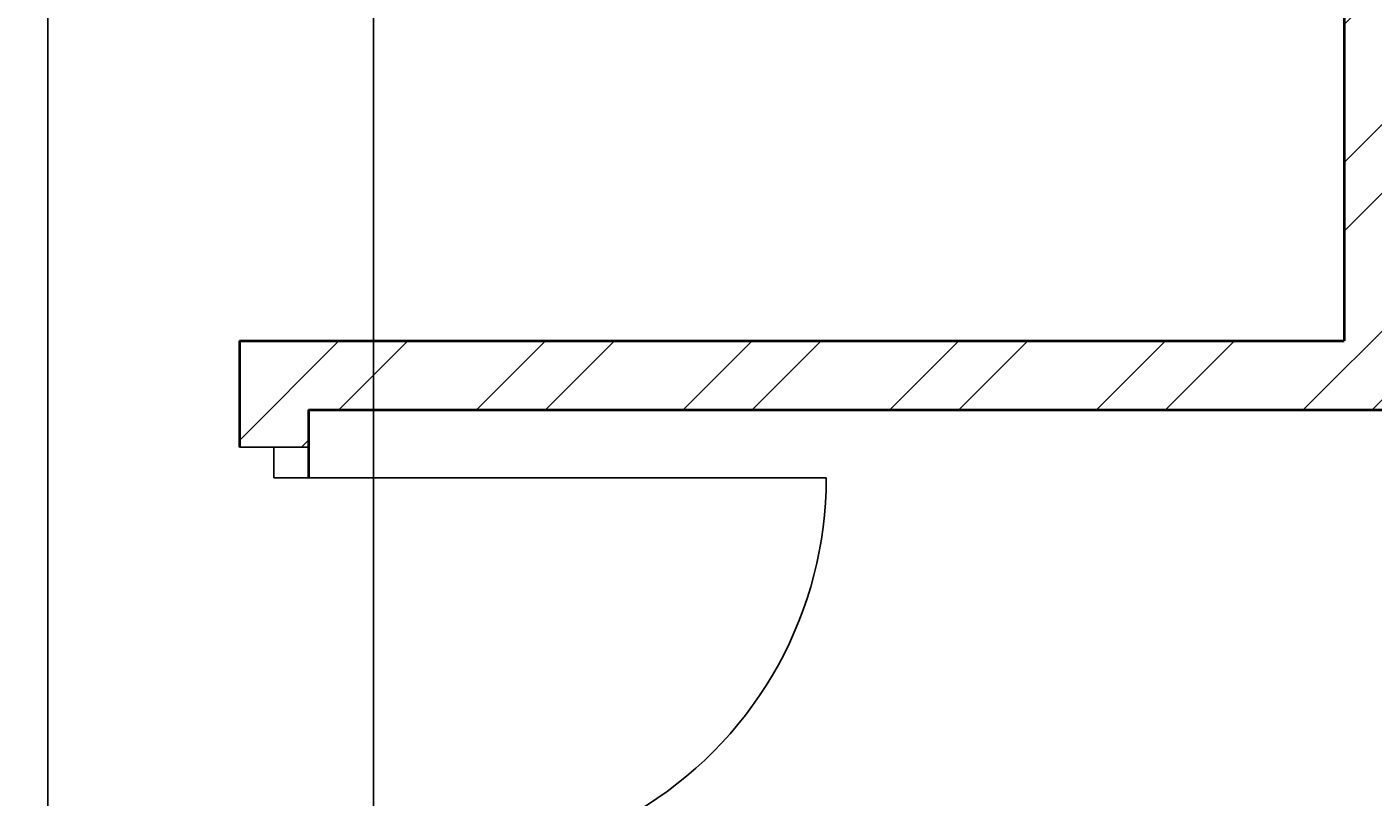
# Model space of a CAD drawing. Units: inches. Extents: x 2063 to 2617, y 1299 to 2210.
# Tile 17 of 22: x 2387 to 2475, y 1839 to 1889. Entities that reach past the tile are written whole.
import ezdxf

# ---------------------------------------------------------------- set-up
doc = ezdxf.new("R2010")
doc.units = ezdxf.units.IN
for name, color, linetype, lineweight in [('A-ANNO-DIMS', 2, 'Continuous', 18), ('A-DOOR', 11, 'Continuous', 25), ('A-WALL', 7, 'Continuous', 40)]:
    doc.layers.add(name, color=color, linetype=linetype, lineweight=lineweight)
doc.layers.add('A-WALL-PATT', color=215, linetype='Continuous', lineweight=13, true_color=0xa953a0)
doc.styles.get("Standard").update_dxf_attribs({"font": 'arial.ttf'})
doc.dimstyles.get("Standard").update_dxf_attribs({"dimtxt": 0.18, "dimasz": 0.18, "dimexe": 0.18, "dimexo": 0.0625, "dimgap": 0.09, "dimtad": 0, "dimtih": 1, "dimtoh": 1, "dimdec": 4, "dimzin": 0, "dimdsep": 46, "dimtxsty": 'Standard', "dimcen": 0.09, "dimadec": 0, "dimazin": 0, "dimtfac": 1, "dimtdec": 4, "dimtofl": 0, "dimtmove": 0, "dimatfit": 3, "dimfxl": 1, "dimtolj": 1, "dimtzin": 0, "dimarcsym": 0})

# ---------------------------------------------------------------- blocks, each defined once
blk = doc.blocks.new('*D55')
at = {"layer": 'A-ANNO-DIMS', "color": 0, "lineweight": -2, "transparency": 16777216}
for p, q in [((2388.15, 1975.75), (2388.15, 1317.702)), ((2409.375, 1975.75), (2409.375, 1317.702)), ((2388.33, 1317.882), (2398.297, 1317.882)), ((2409.195, 1317.882), (2399.229, 1317.882))]:
    blk.add_line(p, q, dxfattribs=at)
at = {"layer": 'A-ANNO-DIMS', "color": 0, "transparency": 16777216}
for points in [[(2388.33, 1317.912), (2388.33, 1317.852), (2388.15, 1317.882)], [(2409.195, 1317.912), (2409.195, 1317.852), (2409.375, 1317.882)]]:
    blk.add_solid(points, dxfattribs=at)
at = {"layer": 'Defpoints', "color": 0, "transparency": 16777216}
for p in [(2388.15, 1975.812), (2409.375, 1975.812), (2409.375, 1317.882)]:
    blk.add_point(p, dxfattribs=at)
at = {"layer": 'A-ANNO-DIMS', "color": 0, "transparency": 16777216, "insert": (2398.763, 1317.882), "char_height": 0.18, "attachment_point": 5}
blk.add_mtext('\\A1;21.225', dxfattribs=at)

msp = doc.modelspace()

# ---------------------------------------------------------------- hatches: boundary and pattern name
at = {"layer": 'A-WALL-PATT'}
h = msp.add_hatch(dxfattribs=at)
h.set_pattern_fill('ANSI32', color=256)
h.paths.add_polyline_path([(2553.6442, 2128.8122), (2511.1703, 2128.8122), (2511.1703, 2124.3122), (2549.1442, 2124.3122), (2549.1442, 2095.662), (2553.6442, 2095.662)])
h.paths.add_polyline_path([(2553.6442, 2035.662), (2549.1442, 2035.662), (2549.1442, 1980.3122), (2503.7214, 1980.3122), (2503.7214, 1975.8122), (2549.1442, 1975.8122), (2549.1442, 1962.9693), (2553.6442, 1962.9693)])
h.paths.add_polyline_path([(2553.6442, 1938.9693), (2549.1442, 1938.9693), (2549.1442, 1927.8122), (2477.1442, 1927.8122), (2477.1442, 1975.8122), (2481.2918, 1975.8122), (2481.2918, 1980.3122), (2453.2648, 1980.3122), (2453.2648, 1975.8122), (2472.6442, 1975.8122), (2472.6442, 1868.3122), (2400.6442, 1868.3122), (2400.6442, 1861.3782), (2405.1442, 1861.3782), (2405.1442, 1863.8122), (2480.9699, 1863.8122), (2480.9699, 1866.0622), (2480.9699, 1868.3122), (2477.1442, 1868.3122), (2477.1442, 1923.3122), (2549.1442, 1923.3122), (2549.1442, 1908.8504), (2553.6442, 1908.8504)])
h.paths.add_polyline_path([(2553.6442, 1884.8504), (2549.1442, 1884.8504), (2549.1442, 1868.3122), (2501.0636, 1868.3122), (2501.0636, 1863.8122), (2549.1442, 1863.8122), (2549.1442, 1826.0298), (2553.6442, 1826.0298)])
h.paths.add_polyline_path([(2388.1504, 1980.3122), (2340.6442, 1980.3122), (2340.6442, 2124.3122), (2358.7501, 2124.3122), (2358.7501, 2128.8122), (2316.3482, 2128.8122), (2316.3482, 2124.3122), (2336.1442, 2124.3122), (2336.1442, 1980.3122), (2289.1737, 1980.3122), (2289.1737, 1975.8122), (2336.1442, 1975.8122), (2336.1442, 1619.3122), (2333.1433, 1619.3122), (2333.1433, 1614.8122), (2344.1671, 1614.8122), (2344.1671, 1617.0622), (2344.1671, 1619.3122), (2340.6442, 1619.3122), (2340.6442, 1975.8122), (2388.1504, 1975.8122), (2388.1504, 1978.0622)])
h.paths.add_polyline_path([(2290.1442, 1614.8122), (2301.4594, 1614.8122), (2301.4594, 1617.0622), (2301.4594, 1619.3122), (2285.6442, 1619.3122), (2285.6442, 1566.8122), (2280.8619, 1566.8122), (2280.8619, 1564.5622), (2280.8619, 1562.3122), (2285.6442, 1562.3122), (2285.6442, 1442.3122), (2281.7879, 1442.3122), (2281.7879, 1437.8122), (2285.6442, 1437.8122), (2285.6442, 1401.8122), (2290.1442, 1401.8122)])
h.paths.add_polyline_path([(2549.1442, 1731.8122), (2405.1442, 1731.8122), (2405.1442, 1834.4638), (2402.8942, 1834.4638), (2400.6442, 1834.4638), (2400.6442, 1727.3122), (2549.1442, 1727.3122)])
h.paths.add_polyline_path([(2553.6442, 1766.0298), (2551.3942, 1766.0298), (2549.1442, 1766.0298), (2549.1442, 1686.7767), (2553.6442, 1686.7767)])
h.paths.add_polyline_path([(2553.6442, 1638.7767), (2551.3942, 1638.7767), (2549.1442, 1638.7767), (2549.1442, 1619.3122), (2448.6442, 1619.3122), (2448.6442, 1610.5671), (2450.8942, 1610.5671), (2453.1442, 1610.5671), (2453.1442, 1614.8122), (2549.1442, 1614.8122), (2549.1442, 1601.6421), (2553.6442, 1601.6421)])
h.paths.add_polyline_path([(2553.6442, 1577.6421), (2551.3942, 1577.6421), (2549.1442, 1577.6421), (2549.1442, 1566.8122), (2453.1442, 1566.8122), (2453.1442, 1591.5045), (2451.0335, 1591.5045), (2448.6442, 1591.5045), (2448.6442, 1566.8122), (2434.0475, 1566.8122), (2434.0475, 1562.3122), (2549.1442, 1562.3122), (2549.1442, 1533.48), (2553.6442, 1533.48)])
h.paths.add_polyline_path([(2553.6442, 1473.48), (2549.1442, 1473.48), (2549.1442, 1442.3122), (2502.6258, 1442.3122), (2502.6258, 1437.8122), (2549.1442, 1437.8122), (2549.1442, 1401.8122), (2553.6442, 1401.8122)])
h.paths.add_polyline_path([(2395.6442, 1562.3122), (2400.0901, 1562.3122), (2400.0901, 1564.5622), (2400.0901, 1566.8122), (2395.6442, 1566.8122), (2395.6442, 1619.3122), (2379.1127, 1619.3122), (2379.1127, 1614.8122), (2391.1442, 1614.8122), (2391.1442, 1401.8122), (2395.6442, 1401.8122), (2395.6442, 1437.8122), (2399.2425, 1437.8122), (2399.2425, 1440.0622), (2399.2425, 1442.3122), (2395.6442, 1442.3122)])
h.paths.add_polyline_path([(2442.6258, 1442.3122), (2419.6262, 1442.3122), (2419.6262, 1437.8122), (2442.6258, 1437.8122), (2442.6258, 1440.0622)])
h.paths.add_polyline_path([(2127.6442, 1480.2532), (2125.3942, 1480.2532), (2123.1442, 1480.2532), (2123.1442, 1401.8122), (2127.6442, 1401.8122), (2127.6442, 1437.8122), (2145.1538, 1437.8122), (2145.1538, 1440.0622), (2145.1538, 1442.3122), (2127.6442, 1442.3122)])
h.paths.add_polyline_path([(2259.809, 1442.3122), (2205.1538, 1442.3122), (2205.1538, 1437.8122), (2259.809, 1437.8122), (2259.809, 1440.0622)])
h.paths.add_polyline_path([(2127.6442, 1659.7652), (2123.1442, 1659.7652), (2123.1442, 1605.5161), (2125.3942, 1605.5161), (2127.6442, 1605.5161), (2127.6442, 1614.8122), (2223.6442, 1614.8122), (2223.6442, 1611.2723), (2228.1442, 1611.2723), (2228.1442, 1619.3122), (2127.6442, 1619.3122)])
h.paths.add_polyline_path([(2244.8673, 1566.8122), (2228.1442, 1566.8122), (2228.1442, 1590.8122), (2225.8942, 1590.8122), (2223.6442, 1590.8122), (2223.6442, 1566.8122), (2127.6442, 1566.8122), (2127.6442, 1581.5161), (2123.1442, 1581.5161), (2123.1442, 1540.2532), (2127.6442, 1540.2532), (2127.6442, 1562.3122), (2244.8673, 1562.3122), (2244.8673, 1564.5622)])
h.paths.add_polyline_path([(2172.5174, 1868.3122), (2127.6442, 1868.3122), (2127.6442, 1886.5833), (2123.1442, 1886.5833), (2123.1442, 1832.6633), (2127.6442, 1832.6633), (2127.6442, 1863.8122), (2172.5174, 1863.8122), (2172.5174, 1866.0622)])
h.paths.add_polyline_path([(2276.1442, 1868.3122), (2204.1442, 1868.3122), (2204.1442, 1923.3122), (2204.1442, 1975.8122), (2224.8362, 1975.8122), (2224.8362, 1978.1097), (2224.8362, 1980.3122), (2195.0729, 1980.3122), (2195.0729, 1978.0622), (2195.0729, 1975.8122), (2199.6442, 1975.8122), (2199.6442, 1927.8122), (2127.6442, 1927.8122), (2127.6442, 1942.3492), (2123.1442, 1942.3492), (2123.1442, 1910.5833), (2127.6442, 1910.5833), (2127.6442, 1923.3122), (2199.6442, 1923.3122), (2199.6442, 1868.3122), (2194.8228, 1868.3122), (2194.8228, 1864.7337), (2194.8228, 1863.8122), (2271.6442, 1863.8122), (2271.6442, 1860.0507), (2276.1442, 1860.0507)])
h.paths.add_polyline_path([(2276.1442, 1829.994), (2273.8942, 1829.994), (2271.6442, 1829.994), (2271.6442, 1731.8122), (2127.6442, 1731.8122), (2127.6442, 1772.6633), (2123.1442, 1772.6633), (2123.1442, 1707.7652), (2127.6442, 1707.7652), (2127.6442, 1727.3122), (2276.1442, 1727.3122)])
h.paths.add_polyline_path([(2127.6442, 2022.1152), (2123.1442, 2022.1152), (2123.1442, 1966.3492), (2127.6442, 1966.3492), (2127.6442, 1975.8122), (2174.2082, 1975.8122), (2174.2082, 1978.0622), (2174.2082, 1980.3122), (2127.6442, 1980.3122)])
h.paths.add_polyline_path([(2361.9755, 1678.588), (2398.4558, 1678.588), (2398.4558, 1697.2453), (2361.9755, 1697.2453)], flags=9)
h.paths.add_polyline_path([(2351.5397, 1780.4072), (2386.1987, 1780.4072), (2386.1987, 1790.7107), (2351.5397, 1790.7107)], flags=25)
h.paths.add_polyline_path([(2350.6753, 1940.9321), (2387.6024, 1940.9321), (2387.6024, 1959.5894), (2350.6753, 1959.5894)], flags=25)
h.paths.add_polyline_path([(2254.9545, 1684.638), (2295.0943, 1684.638), (2295.0943, 1703.2953), (2254.9545, 1703.2953)], flags=9)
h.paths.add_polyline_path([(2282.4946, 1782.4438), (2317.1535, 1782.4438), (2317.1535, 1792.7474), (2282.4946, 1792.7474)], flags=9)
h.paths.add_polyline_path([(2270.327, 1939.2854), (2307.254, 1939.2854), (2307.254, 1957.9428), (2270.327, 1957.9428)], flags=9)

# ---------------------------------------------------------------- linework, layer by layer
at = {"layer": 'A-DOOR'}
for p, q in [((2400.6442, 1861.3782), (2405.1442, 1861.3782)), ((2405.1442, 1861.3782), (2402.8942, 1861.3782)), ((2402.8942, 1861.3782), (2402.8942, 1859.3782)), ((2402.8942, 1859.3782), (2438.8942, 1859.3782))]:
    msp.add_line(p, q, dxfattribs=at)
msp.add_arc((2413.6016, 1859.3782), 25.2926, 244.954413, 0, dxfattribs=at)
at = {"layer": 'A-WALL'}
for p, q in [((2472.6442, 1975.8122), (2472.6442, 1868.3122)), ((2400.6442, 1868.3122), (2400.6442, 1861.3782)), ((2400.6442, 1868.3122), (2472.6442, 1868.3122)), ((2405.1442, 1863.8122), (2405.1442, 1859.3782)), ((2405.1442, 1863.8122), (2480.9699, 1863.8122))]:
    msp.add_line(p, q, dxfattribs=at)

# ---------------------------------------------------------------- dimensions: what is measured, and where the dimension line sits
at = {"layer": 'A-ANNO-DIMS'}
dim = msp.add_linear_dim(base=(2409.375, 1317.8821), p1=(2388.1504, 1975.8122), p2=(2409.375, 1975.8122), dimstyle='Standard', override={"dimdec": 3, "dimlfac": 1, "dimrnd": 0, "dimzin": 0, "dimdsep": 46, "dimlunit": 2}, dxfattribs=at)
dim.commit()
dim.dimension.update_dxf_attribs({"geometry": '*D55', "text_midpoint": (2398.7627, 1317.8821)})

doc.saveas('drawing.dxf')
